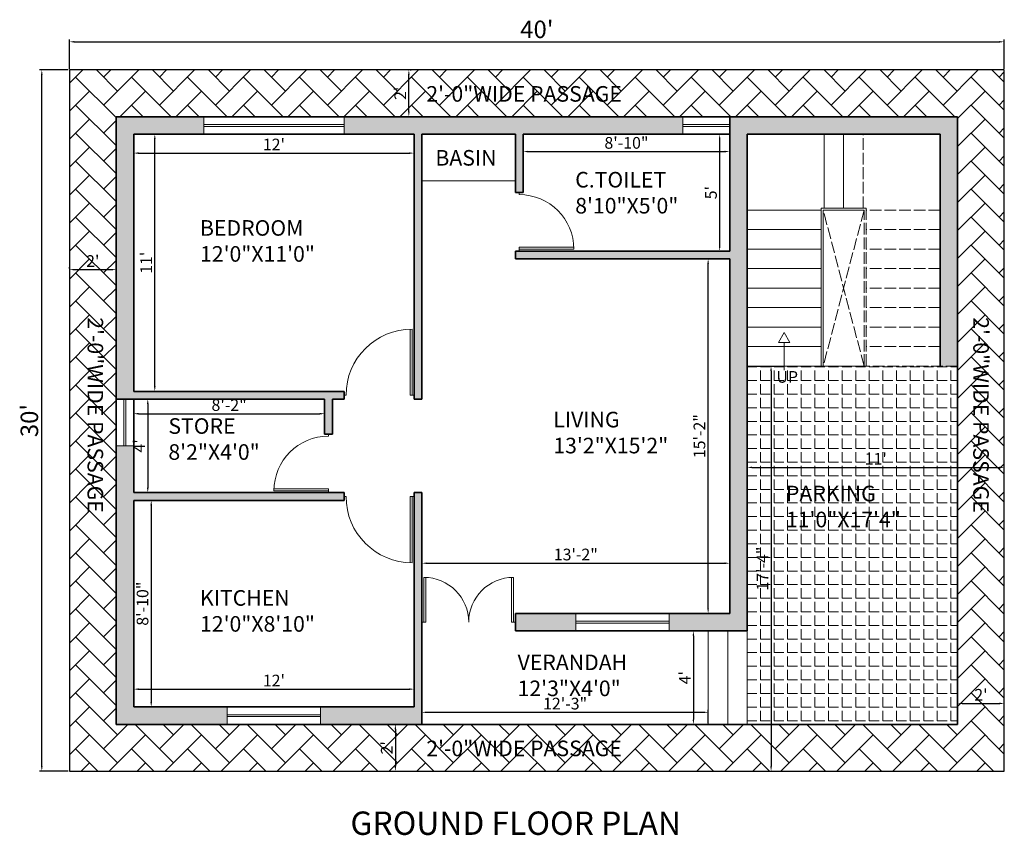
# Model space of a CAD drawing. Units: inches. Extents: x 1947 to 4744, y 610 to 1869.
# Tile 8 of 8: x 4239 to 4744, y 1450 to 1869. Entities that reach past the tile are written whole.
import ezdxf

# ---------------------------------------------------------------- set-up
doc = ezdxf.new("R2010")
doc.units = ezdxf.units.IN
doc.linetypes.add('ACAD_ISO02W100', pattern=[15, 12, -3])
for name, color, linetype, lineweight in [('A-ANNO-DIMS', 2, 'Continuous', 18), ('A-ANNO-SYMB', 2, 'Continuous', 18), ('A-ANNO-TEXT', 7, 'Continuous', 18), ('A-ANNO-TITL', 7, 'Continuous', 35), ('A-AREA-IDEN', 7, 'Continuous', 18), ('A-DOOR', 3, 'Continuous', 18), ('A-FLOR-FIXT', 9, 'Continuous', 18), ('A-FLOR-STRS', 7, 'Continuous', 18), ('A-FLOR-STRS-OVHD', 7, 'ACAD_ISO02W100', 13), ('A-GLAZ', 4, 'Continuous', 18), ('A-WALL', 7, 'Continuous', 35), ('C-PROP', 8, 'Continuous', 25)]:
    doc.layers.add(name, color=color, linetype=linetype, lineweight=lineweight)
doc.layers.add('A-FLOR-PATT', color=251, linetype='Continuous', lineweight=13, true_color=0x636466)
doc.layers.add('A-WALL-PATT', color=18, linetype='Continuous', lineweight=13, true_color=0x000000)
doc.styles.get("Standard").update_dxf_attribs({"font": 'arial.ttf'})
doc.dimstyles.new('ISO-25', dxfattribs={"dimtxt": 9, "dimasz": 2.5, "dimexe": 1.25, "dimexo": 0.625, "dimtad": 1, "dimdec": 1, "dimlunit": 3, "dimtxsty": 'Standard', "dimcen": 2.5, "dimadec": 0, "dimazin": 0, "dimtfac": 1, "dimtdec": 1, "dimtmove": 0, "dimatfit": 3, "dimfxl": 1, "dimarcsym": 0})

# ---------------------------------------------------------------- blocks, each defined once
blk = doc.blocks.new('1')
for p, q in [((4267.36, 1627.82), (4267.36, 1650.82)), ((4268.36, 1627.82), (4268.36, 1650.82)), ((4312.36, 1627.82), (4312.36, 1650.82)), ((4313.36, 1627.82), (4313.36, 1650.82)), ((4266.36, 1627.82), (4268.36, 1627.82)), ((4314.36, 1627.82), (4312.36, 1627.82))]:
    blk.add_line(p, q)
at = {"ltscale": 0.5}
for centre, start, end in [((4267.36, 1627.82), 0, 90), ((4313.36, 1627.82), 90, 180)]:
    blk.add_arc(centre, 23, start, end, dxfattribs=at)
blk = doc.blocks.new('2')
for p, q in [((4319.45, 1679.18), (4319.45, 1713.18)), ((4320.45, 1679.18), (4320.45, 1713.18)), ((4318.45, 1679.18), (4320.45, 1679.18)), ((4353.45, 1679.18), (4354.45, 1679.18))]:
    blk.add_line(p, q)
at = {"ltscale": 0.5}
blk.add_arc((4319.45, 1679.18), 34, 0, 90, dxfattribs=at)
blk = doc.blocks.new('4')
for p, q in [((3808.6, 1693.11), (3808.6, 1721.11)), ((3809.6, 1693.11), (3809.6, 1721.11)), ((3807.6, 1693.11), (3809.6, 1693.11)), ((3836.6, 1693.11), (3837.6, 1693.11))]:
    blk.add_line(p, q)
at = {"ltscale": 0.5}
blk.add_arc((3808.6, 1693.11), 28, 0, 90, dxfattribs=at)
blk = doc.blocks.new('*D11')
at = {"layer": 'A-ANNO-DIMS', "color": 0, "lineweight": -2, "transparency": 16777216}
for p, q in [((4263.57, 1842.83), (4248.77, 1842.83)), ((4250.02, 1485.33), (4250.02, 1840.33)), ((4263.57, 1482.83), (4248.77, 1482.83))]:
    blk.add_line(p, q, dxfattribs=at)
at = {"layer": 'A-ANNO-DIMS', "color": 0, "transparency": 16777216}
for points in [[(4249.6, 1840.33), (4250.44, 1840.33), (4250.02, 1842.83)], [(4249.6, 1485.33), (4250.44, 1485.33), (4250.02, 1482.83)]]:
    blk.add_solid(points, dxfattribs=at)
at = {"layer": 'Defpoints', "color": 0, "transparency": 16777216}
for p in [(4250.02, 1842.83), (4264.19, 1842.83), (4264.19, 1482.83)]:
    blk.add_point(p, dxfattribs=at)
at = {"layer": 'A-ANNO-DIMS', "color": 0, "transparency": 16777216, "insert": (4244.8, 1662.83), "char_height": 9, "attachment_point": 5, "rotation": 90}
blk.add_mtext("30'", dxfattribs=at)
blk = doc.blocks.new('*D12')
at = {"layer": 'A-ANNO-DIMS', "color": 0, "lineweight": -2, "transparency": 16777216}
for p, q in [((4264.19, 1843.45), (4264.19, 1858.52)), ((4266.69, 1857.27), (4741.69, 1857.27)), ((4744.19, 1843.45), (4744.19, 1858.52))]:
    blk.add_line(p, q, dxfattribs=at)
at = {"layer": 'A-ANNO-DIMS', "color": 0, "transparency": 16777216}
for points in [[(4266.69, 1857.68), (4266.69, 1856.85), (4264.19, 1857.27)], [(4741.69, 1857.68), (4741.69, 1856.85), (4744.19, 1857.27)]]:
    blk.add_solid(points, dxfattribs=at)
at = {"layer": 'Defpoints', "color": 0, "transparency": 16777216}
for p in [(4744.19, 1857.27), (4264.19, 1842.83), (4744.19, 1842.83)]:
    blk.add_point(p, dxfattribs=at)
at = {"layer": 'A-ANNO-DIMS', "color": 0, "transparency": 16777216, "insert": (4504.19, 1862.49), "char_height": 9, "attachment_point": 5}
blk.add_mtext("40'", dxfattribs=at)
blk = doc.blocks.new('*D17')
at = {"layer": 'A-ANNO-DIMS', "color": 0, "lineweight": -2, "transparency": 16777216}
for p, q in [((4297.82, 1809.83), (4309.28, 1809.83)), ((4308.03, 1680.33), (4308.03, 1807.33)), ((4297.82, 1677.83), (4309.28, 1677.83))]:
    blk.add_line(p, q, dxfattribs=at)
at = {"layer": 'A-ANNO-DIMS', "color": 0, "transparency": 16777216}
for points in [[(4307.62, 1807.33), (4308.45, 1807.33), (4308.03, 1809.83)], [(4307.62, 1680.33), (4308.45, 1680.33), (4308.03, 1677.83)]]:
    blk.add_solid(points, dxfattribs=at)
at = {"layer": 'Defpoints', "color": 0, "transparency": 16777216}
for p in [(4297.19, 1809.83), (4308.03, 1809.83), (4297.19, 1677.83)]:
    blk.add_point(p, dxfattribs=at)
at = {"layer": 'A-ANNO-DIMS', "color": 0, "transparency": 16777216, "insert": (4304.4, 1743.83), "char_height": 6, "attachment_point": 5, "rotation": 90}
blk.add_mtext("11'", dxfattribs=at)
blk = doc.blocks.new('*D18')
at = {"layer": 'A-ANNO-DIMS', "color": 0, "lineweight": -2, "transparency": 16777216}
for p, q in [((4297.19, 1809.2), (4297.19, 1798.88)), ((4441.19, 1809.2), (4441.19, 1798.88)), ((4299.69, 1800.13), (4438.69, 1800.13))]:
    blk.add_line(p, q, dxfattribs=at)
at = {"layer": 'A-ANNO-DIMS', "color": 0, "transparency": 16777216}
for points in [[(4299.69, 1800.54), (4299.69, 1799.71), (4297.19, 1800.13)], [(4438.69, 1800.54), (4438.69, 1799.71), (4441.19, 1800.13)]]:
    blk.add_solid(points, dxfattribs=at)
at = {"layer": 'Defpoints', "color": 0, "transparency": 16777216}
for p in [(4297.19, 1809.83), (4441.19, 1809.83), (4441.19, 1800.13)]:
    blk.add_point(p, dxfattribs=at)
at = {"layer": 'A-ANNO-DIMS', "color": 0, "transparency": 16777216, "insert": (4369.19, 1803.76), "char_height": 6, "attachment_point": 5}
blk.add_mtext("12'", dxfattribs=at)
blk = doc.blocks.new('*D19')
at = {"layer": 'A-ANNO-DIMS', "color": 0, "lineweight": -2, "transparency": 16777216}
for p, q in [((4497.19, 1809.2), (4497.19, 1799.67)), ((4603.19, 1809.2), (4603.19, 1799.67)), ((4499.69, 1800.92), (4600.69, 1800.92))]:
    blk.add_line(p, q, dxfattribs=at)
at = {"layer": 'A-ANNO-DIMS', "color": 0, "transparency": 16777216}
for points in [[(4499.69, 1801.34), (4499.69, 1800.5), (4497.19, 1800.92)], [(4600.69, 1801.34), (4600.69, 1800.5), (4603.19, 1800.92)]]:
    blk.add_solid(points, dxfattribs=at)
at = {"layer": 'Defpoints', "color": 0, "transparency": 16777216}
for p in [(4497.19, 1809.83), (4603.19, 1809.83), (4603.19, 1800.92)]:
    blk.add_point(p, dxfattribs=at)
at = {"layer": 'A-ANNO-DIMS', "color": 0, "transparency": 16777216, "insert": (4550.19, 1804.61), "char_height": 6, "attachment_point": 5}
blk.add_mtext('8\'-10"', dxfattribs=at)
blk = doc.blocks.new('*D20')
at = {"layer": 'A-ANNO-DIMS', "color": 0, "lineweight": -2, "transparency": 16777216}
for p, q in [((4602.57, 1809.83), (4596.8, 1809.83)), ((4598.05, 1807.33), (4598.05, 1752.33)), ((4602.57, 1749.83), (4596.8, 1749.83))]:
    blk.add_line(p, q, dxfattribs=at)
at = {"layer": 'A-ANNO-DIMS', "color": 0, "transparency": 16777216}
for points in [[(4597.63, 1807.33), (4598.46, 1807.33), (4598.05, 1809.83)], [(4597.63, 1752.33), (4598.46, 1752.33), (4598.05, 1749.83)]]:
    blk.add_solid(points, dxfattribs=at)
at = {"layer": 'Defpoints', "color": 0, "transparency": 16777216}
for p in [(4603.19, 1809.83), (4598.05, 1749.83), (4603.19, 1749.83)]:
    blk.add_point(p, dxfattribs=at)
at = {"layer": 'A-ANNO-DIMS', "color": 0, "transparency": 16777216, "insert": (4594.37, 1779.83), "char_height": 6, "attachment_point": 5, "rotation": 90}
blk.add_mtext("5'", dxfattribs=at)
blk = doc.blocks.new('*D21')
at = {"layer": 'A-ANNO-DIMS', "color": 0, "lineweight": -2, "transparency": 16777216}
for p, q in [((4297.82, 1673.83), (4305.68, 1673.83)), ((4304.43, 1671.33), (4304.43, 1628.33)), ((4297.82, 1625.83), (4305.68, 1625.83))]:
    blk.add_line(p, q, dxfattribs=at)
at = {"layer": 'A-ANNO-DIMS', "color": 0, "transparency": 16777216}
for points in [[(4304.01, 1671.33), (4304.85, 1671.33), (4304.43, 1673.83)], [(4304.01, 1628.33), (4304.85, 1628.33), (4304.43, 1625.83)]]:
    blk.add_solid(points, dxfattribs=at)
at = {"layer": 'Defpoints', "color": 0, "transparency": 16777216}
for p in [(4297.19, 1673.83), (4297.19, 1625.83), (4304.43, 1625.83)]:
    blk.add_point(p, dxfattribs=at)
at = {"layer": 'A-ANNO-DIMS', "color": 0, "transparency": 16777216, "insert": (4300.8, 1649.83), "char_height": 6, "attachment_point": 5, "rotation": 90}
blk.add_mtext("4'", dxfattribs=at)
blk = doc.blocks.new('*D22')
at = {"layer": 'A-ANNO-DIMS', "color": 0, "lineweight": -2, "transparency": 16777216}
for p, q in [((4297.19, 1673.2), (4297.19, 1665.09)), ((4395.19, 1673.2), (4395.19, 1665.09)), ((4299.69, 1666.34), (4392.69, 1666.34))]:
    blk.add_line(p, q, dxfattribs=at)
at = {"layer": 'A-ANNO-DIMS', "color": 0, "transparency": 16777216}
for points in [[(4299.69, 1666.76), (4299.69, 1665.93), (4297.19, 1666.34)], [(4392.69, 1666.76), (4392.69, 1665.93), (4395.19, 1666.34)]]:
    blk.add_solid(points, dxfattribs=at)
at = {"layer": 'Defpoints', "color": 0, "transparency": 16777216}
for p in [(4297.19, 1673.83), (4395.19, 1673.83), (4395.19, 1666.34)]:
    blk.add_point(p, dxfattribs=at)
at = {"layer": 'A-ANNO-DIMS', "color": 0, "transparency": 16777216, "insert": (4346.19, 1670.03), "char_height": 6, "attachment_point": 5}
blk.add_mtext('8\'-2"', dxfattribs=at)
blk = doc.blocks.new('*D23')
at = {"layer": 'A-ANNO-DIMS', "color": 0, "lineweight": -2, "transparency": 16777216}
for p, q in [((4297.82, 1621.83), (4307.45, 1621.83)), ((4306.2, 1619.33), (4306.2, 1518.33)), ((4297.82, 1515.83), (4307.45, 1515.83))]:
    blk.add_line(p, q, dxfattribs=at)
at = {"layer": 'A-ANNO-DIMS', "color": 0, "transparency": 16777216}
for points in [[(4305.78, 1619.33), (4306.61, 1619.33), (4306.2, 1621.83)], [(4305.78, 1518.33), (4306.61, 1518.33), (4306.2, 1515.83)]]:
    blk.add_solid(points, dxfattribs=at)
at = {"layer": 'Defpoints', "color": 0, "transparency": 16777216}
for p in [(4297.19, 1621.83), (4297.19, 1515.83), (4306.2, 1515.83)]:
    blk.add_point(p, dxfattribs=at)
at = {"layer": 'A-ANNO-DIMS', "color": 0, "transparency": 16777216, "insert": (4302.51, 1568.83), "char_height": 6, "attachment_point": 5, "rotation": 90}
blk.add_mtext('8\'-10"', dxfattribs=at)
blk = doc.blocks.new('*D24')
at = {"layer": 'A-ANNO-DIMS', "color": 0, "lineweight": -2, "transparency": 16777216}
for p, q in [((4297.19, 1516.45), (4297.19, 1526.2)), ((4299.69, 1524.95), (4438.69, 1524.95)), ((4441.19, 1516.45), (4441.19, 1526.2))]:
    blk.add_line(p, q, dxfattribs=at)
at = {"layer": 'A-ANNO-DIMS', "color": 0, "transparency": 16777216}
for points in [[(4299.69, 1525.37), (4299.69, 1524.53), (4297.19, 1524.95)], [(4438.69, 1525.37), (4438.69, 1524.53), (4441.19, 1524.95)]]:
    blk.add_solid(points, dxfattribs=at)
at = {"layer": 'Defpoints', "color": 0, "transparency": 16777216}
for p in [(4441.19, 1524.95), (4297.19, 1515.83), (4441.19, 1515.83)]:
    blk.add_point(p, dxfattribs=at)
at = {"layer": 'A-ANNO-DIMS', "color": 0, "transparency": 16777216, "insert": (4369.19, 1528.59), "char_height": 6, "attachment_point": 5}
blk.add_mtext("12'", dxfattribs=at)
blk = doc.blocks.new('*D25')
at = {"layer": 'A-ANNO-DIMS', "color": 0, "lineweight": -2, "transparency": 16777216}
for p, q in [((4445.19, 1588.97), (4445.19, 1588.35)), ((4447.69, 1589.6), (4600.69, 1589.6)), ((4603.19, 1590.22), (4603.19, 1590.85))]:
    blk.add_line(p, q, dxfattribs=at)
at = {"layer": 'A-ANNO-DIMS', "color": 0, "transparency": 16777216}
for points in [[(4447.69, 1590.01), (4447.69, 1589.18), (4445.19, 1589.6)], [(4600.69, 1590.01), (4600.69, 1589.18), (4603.19, 1589.6)]]:
    blk.add_solid(points, dxfattribs=at)
at = {"layer": 'Defpoints', "color": 0, "transparency": 16777216}
for p in [(4445.19, 1589.6), (4603.19, 1589.6), (4603.19, 1589.6)]:
    blk.add_point(p, dxfattribs=at)
at = {"layer": 'A-ANNO-DIMS', "color": 0, "transparency": 16777216, "insert": (4524.19, 1593.29), "char_height": 6, "attachment_point": 5}
blk.add_mtext('13\'-2"', dxfattribs=at)
blk = doc.blocks.new('*D26')
at = {"layer": 'A-ANNO-DIMS', "color": 0, "lineweight": -2, "transparency": 16777216}
for p, q in [((4602.57, 1745.83), (4590.88, 1745.83)), ((4592.13, 1566.33), (4592.13, 1743.33)), ((4602.57, 1563.83), (4590.88, 1563.83))]:
    blk.add_line(p, q, dxfattribs=at)
at = {"layer": 'A-ANNO-DIMS', "color": 0, "transparency": 16777216}
for points in [[(4591.71, 1743.33), (4592.54, 1743.33), (4592.13, 1745.83)], [(4591.71, 1566.33), (4592.54, 1566.33), (4592.13, 1563.83)]]:
    blk.add_solid(points, dxfattribs=at)
at = {"layer": 'Defpoints', "color": 0, "transparency": 16777216}
for p in [(4592.13, 1745.83), (4603.19, 1745.83), (4603.19, 1563.83)]:
    blk.add_point(p, dxfattribs=at)
at = {"layer": 'A-ANNO-DIMS', "color": 0, "transparency": 16777216, "insert": (4588.44, 1654.83), "char_height": 6, "attachment_point": 5, "rotation": 90}
blk.add_mtext('15\'-2"', dxfattribs=at)
blk = doc.blocks.new('*D27')
at = {"layer": 'A-ANNO-DIMS', "color": 0, "lineweight": -2, "transparency": 16777216}
for p, q in [((4432.16, 1506.83), (4432.78, 1506.83)), ((4431.53, 1504.33), (4431.53, 1485.33)), ((4432.16, 1482.83), (4432.78, 1482.83))]:
    blk.add_line(p, q, dxfattribs=at)
at = {"layer": 'A-ANNO-DIMS', "color": 0, "transparency": 16777216}
for points in [[(4431.12, 1504.33), (4431.95, 1504.33), (4431.53, 1506.83)], [(4431.12, 1485.33), (4431.95, 1485.33), (4431.53, 1482.83)]]:
    blk.add_solid(points, dxfattribs=at)
at = {"layer": 'Defpoints', "color": 0, "transparency": 16777216}
for p in [(4431.53, 1506.83), (4431.53, 1482.83), (4431.53, 1482.83)]:
    blk.add_point(p, dxfattribs=at)
at = {"layer": 'A-ANNO-DIMS', "color": 0, "transparency": 16777216, "insert": (4427.9, 1494.83), "char_height": 6, "attachment_point": 5, "rotation": 90}
blk.add_mtext("2'", dxfattribs=at)
blk = doc.blocks.new('*D28')
at = {"layer": 'A-ANNO-DIMS', "color": 0, "lineweight": -2, "transparency": 16777216}
for p, q in [((4264.19, 1740.93), (4264.19, 1741.56)), ((4266.69, 1740.31), (4285.69, 1740.31)), ((4288.19, 1740.93), (4288.19, 1741.56))]:
    blk.add_line(p, q, dxfattribs=at)
at = {"layer": 'A-ANNO-DIMS', "color": 0, "transparency": 16777216}
for points in [[(4266.69, 1740.72), (4266.69, 1739.89), (4264.19, 1740.31)], [(4285.69, 1740.72), (4285.69, 1739.89), (4288.19, 1740.31)]]:
    blk.add_solid(points, dxfattribs=at)
at = {"layer": 'Defpoints', "color": 0, "transparency": 16777216}
for p in [(4264.19, 1740.31), (4288.19, 1740.31), (4288.19, 1740.31)]:
    blk.add_point(p, dxfattribs=at)
at = {"layer": 'A-ANNO-DIMS', "color": 0, "transparency": 16777216, "insert": (4276.19, 1743.94), "char_height": 6, "attachment_point": 5}
blk.add_mtext("2'", dxfattribs=at)
blk = doc.blocks.new('*D29')
at = {"layer": 'A-ANNO-DIMS', "color": 0, "lineweight": -2, "transparency": 16777216}
for p, q in [((4438.47, 1821.33), (4438.47, 1840.33)), ((4439.1, 1842.83), (4439.72, 1842.83)), ((4439.1, 1818.83), (4439.72, 1818.83))]:
    blk.add_line(p, q, dxfattribs=at)
at = {"layer": 'A-ANNO-DIMS', "color": 0, "transparency": 16777216}
for points in [[(4438.06, 1840.33), (4438.89, 1840.33), (4438.47, 1842.83)], [(4438.06, 1821.33), (4438.89, 1821.33), (4438.47, 1818.83)]]:
    blk.add_solid(points, dxfattribs=at)
at = {"layer": 'Defpoints', "color": 0, "transparency": 16777216}
for p in [(4438.47, 1842.83), (4438.47, 1842.83), (4438.47, 1818.83)]:
    blk.add_point(p, dxfattribs=at)
at = {"layer": 'A-ANNO-DIMS', "color": 0, "transparency": 16777216, "insert": (4434.84, 1830.83), "char_height": 6, "attachment_point": 5, "rotation": 90}
blk.add_mtext("2'", dxfattribs=at)
blk = doc.blocks.new('*D30')
at = {"layer": 'A-ANNO-DIMS', "color": 0, "lineweight": -2, "transparency": 16777216}
for p, q in [((4612.19, 1639.41), (4612.19, 1640.03)), ((4614.69, 1638.78), (4741.69, 1638.78)), ((4744.19, 1639.41), (4744.19, 1640.03))]:
    blk.add_line(p, q, dxfattribs=at)
at = {"layer": 'A-ANNO-DIMS', "color": 0, "transparency": 16777216}
for points in [[(4614.69, 1639.2), (4614.69, 1638.37), (4612.19, 1638.78)], [(4741.69, 1639.2), (4741.69, 1638.37), (4744.19, 1638.78)]]:
    blk.add_solid(points, dxfattribs=at)
at = {"layer": 'Defpoints', "color": 0, "transparency": 16777216}
for p in [(4612.19, 1638.78), (4744.19, 1638.78), (4744.19, 1638.78)]:
    blk.add_point(p, dxfattribs=at)
at = {"layer": 'A-ANNO-DIMS', "color": 0, "transparency": 16777216, "insert": (4678.19, 1642.42), "char_height": 6, "attachment_point": 5}
blk.add_mtext("11'", dxfattribs=at)
blk = doc.blocks.new('*D31')
at = {"layer": 'A-ANNO-DIMS', "color": 0, "lineweight": -2, "transparency": 16777216}
for p, q in [((4612.82, 1690.83), (4625.69, 1690.83)), ((4624.44, 1688.33), (4624.44, 1485.33)), ((4612.82, 1482.83), (4625.69, 1482.83))]:
    blk.add_line(p, q, dxfattribs=at)
at = {"layer": 'A-ANNO-DIMS', "color": 0, "transparency": 16777216}
for points in [[(4624.02, 1688.33), (4624.85, 1688.33), (4624.44, 1690.83)], [(4624.02, 1485.33), (4624.85, 1485.33), (4624.44, 1482.83)]]:
    blk.add_solid(points, dxfattribs=at)
at = {"layer": 'Defpoints', "color": 0, "transparency": 16777216}
for p in [(4612.19, 1690.83), (4612.19, 1482.83), (4624.44, 1482.83)]:
    blk.add_point(p, dxfattribs=at)
at = {"layer": 'A-ANNO-DIMS', "color": 0, "transparency": 16777216, "insert": (4620.8, 1586.83), "char_height": 6, "attachment_point": 5, "rotation": 90}
blk.add_mtext('17\'-4"', dxfattribs=at)
blk = doc.blocks.new('*D32')
at = {"layer": 'A-ANNO-DIMS', "color": 0, "lineweight": -2, "transparency": 16777216}
for p, q in [((4445.19, 1507.45), (4445.19, 1514.31)), ((4447.69, 1513.06), (4589.69, 1513.06)), ((4592.19, 1507.45), (4592.19, 1514.31))]:
    blk.add_line(p, q, dxfattribs=at)
at = {"layer": 'A-ANNO-DIMS', "color": 0, "transparency": 16777216}
for points in [[(4447.69, 1513.48), (4447.69, 1512.64), (4445.19, 1513.06)], [(4589.69, 1513.48), (4589.69, 1512.64), (4592.19, 1513.06)]]:
    blk.add_solid(points, dxfattribs=at)
at = {"layer": 'Defpoints', "color": 0, "transparency": 16777216}
for p in [(4592.19, 1513.06), (4445.19, 1506.83), (4592.19, 1506.83)]:
    blk.add_point(p, dxfattribs=at)
at = {"layer": 'A-ANNO-DIMS', "color": 0, "transparency": 16777216, "insert": (4518.69, 1516.75), "char_height": 6, "attachment_point": 5}
blk.add_mtext('12\'-3"', dxfattribs=at)
blk = doc.blocks.new('*D33')
at = {"layer": 'A-ANNO-DIMS', "color": 0, "lineweight": -2, "transparency": 16777216}
for p, q in [((4591.57, 1554.83), (4583.31, 1554.83)), ((4584.56, 1552.33), (4584.56, 1509.33)), ((4591.57, 1506.83), (4583.31, 1506.83))]:
    blk.add_line(p, q, dxfattribs=at)
at = {"layer": 'A-ANNO-DIMS', "color": 0, "transparency": 16777216}
for points in [[(4584.14, 1552.33), (4584.98, 1552.33), (4584.56, 1554.83)], [(4584.14, 1509.33), (4584.98, 1509.33), (4584.56, 1506.83)]]:
    blk.add_solid(points, dxfattribs=at)
at = {"layer": 'Defpoints', "color": 0, "transparency": 16777216}
for p in [(4592.19, 1554.83), (4584.56, 1506.83), (4592.19, 1506.83)]:
    blk.add_point(p, dxfattribs=at)
at = {"layer": 'A-ANNO-DIMS', "color": 0, "transparency": 16777216, "insert": (4580.94, 1530.83), "char_height": 6, "attachment_point": 5, "rotation": 90}
blk.add_mtext("4'", dxfattribs=at)
blk = doc.blocks.new('*D34')
at = {"layer": 'A-ANNO-DIMS', "color": 0, "lineweight": -2, "transparency": 16777216}
for p, q in [((4720.19, 1507.45), (4720.19, 1518.86)), ((4722.69, 1517.61), (4741.69, 1517.61)), ((4744.19, 1507.45), (4744.19, 1518.86))]:
    blk.add_line(p, q, dxfattribs=at)
at = {"layer": 'A-ANNO-DIMS', "color": 0, "transparency": 16777216}
for points in [[(4722.69, 1518.03), (4722.69, 1517.19), (4720.19, 1517.61)], [(4741.69, 1518.03), (4741.69, 1517.19), (4744.19, 1517.61)]]:
    blk.add_solid(points, dxfattribs=at)
at = {"layer": 'Defpoints', "color": 0, "transparency": 16777216}
for p in [(4744.19, 1517.61), (4720.19, 1506.83), (4744.19, 1506.83)]:
    blk.add_point(p, dxfattribs=at)
at = {"layer": 'A-ANNO-DIMS', "color": 0, "transparency": 16777216, "insert": (4732.19, 1521.25), "char_height": 6, "attachment_point": 5}
blk.add_mtext("2'", dxfattribs=at)
blk = doc.blocks.new('STAIR-DIRECTION')
blk.add_line((2.91, 14.18), (2.91, 0))
blk.add_lwpolyline([(2.91, 19.23), (0, 14.18), (5.83, 14.18)], close=True)

msp = doc.modelspace()

# ---------------------------------------------------------------- hatches: boundary and pattern name
at = {"layer": 'A-FLOR-PATT'}
h = msp.add_hatch(dxfattribs=at)
h.set_pattern_fill('AR-HBONE', color=256, scale=0.1)
h.set_pattern_definition([(45, (574.662, 0), (0, 14.36841), [30.48, -10.16]), (135, (581.846, 7.184), (1e-15, 14.36841), [30.48, -10.16])])
h.paths.add_polyline_path([(4264.19, 1842.83), (4264.19, 1482.83), (4744.19, 1482.83), (4744.19, 1842.83)])
h.paths.add_polyline_path([(4720.19, 1818.83), (4720.19, 1506.83), (4288.19, 1506.83), (4288.19, 1818.83)], flags=16)
h.paths.add_polyline_path([(4297.19, 1625.83), (4405.19, 1625.83), (4405.19, 1621.83), (4297.19, 1621.83), (4297.19, 1515.83), (4393.19, 1515.83), (4393.19, 1510.83), (4345.19, 1510.83), (4345.19, 1515.83), (4297.19, 1515.83)], flags=0)
h.paths.add_polyline_path([(4651.19, 1770.83), (4672.19, 1770.83), (4672.19, 1690.83), (4661.69, 1730.83), (4651.19, 1690.83)], flags=0)
h.paths.add_polyline_path([(4449.88, 1789.16), (4489.33, 1789.16), (4489.33, 1806.24), (4449.88, 1806.24)], flags=8)
h.paths.add_polyline_path([(4445.18, 1485.98), (4558.18, 1485.98), (4558.18, 1503.06), (4445.18, 1503.06)], flags=24)
h.paths.add_polyline_path([(4268.95, 1718.11), (4268.95, 1605.12), (4286.03, 1605.12), (4286.03, 1718.11)], flags=24)
h.paths.add_polyline_path([(4723.69, 1718.11), (4723.69, 1605.12), (4740.77, 1605.12), (4740.77, 1718.11)], flags=24)
h.paths.add_polyline_path([(4445.18, 1821.98), (4558.18, 1821.98), (4558.18, 1839.06), (4445.18, 1839.06)], flags=24)
h.paths.add_polyline_path([(4490.92, 1516.82), (4562.48, 1516.82), (4562.48, 1547.23), (4490.92, 1547.23)], flags=8)
h.paths.add_polyline_path([(4628.7, 1603.48), (4690.57, 1603.48), (4690.57, 1633.9), (4628.7, 1633.9)], flags=8)
h.paths.add_polyline_path([(4312.27, 1638.13), (4362.35, 1638.13), (4362.35, 1668.55), (4312.27, 1668.55)], flags=8)
h.paths.add_polyline_path([(4521.17, 1764.58), (4577.62, 1764.58), (4577.62, 1795), (4521.17, 1795)], flags=8)
h.paths.add_polyline_path([(4509.26, 1641.45), (4571.13, 1641.45), (4571.13, 1671.86), (4509.26, 1671.86)], flags=8)
h.paths.add_polyline_path([(4327.86, 1549.89), (4389.73, 1549.89), (4389.73, 1580.3), (4327.86, 1580.3)], flags=8)
h.paths.add_polyline_path([(4327.86, 1739.82), (4392.11, 1739.82), (4392.11, 1770.24), (4327.86, 1770.24)], flags=8)
h = msp.add_hatch(dxfattribs=at)
h.set_pattern_fill('ANGLE', color=256)
h.set_pattern_definition([(0, (574.662, 0), (0, 6.985), [5.08, -1.905]), (90, (574.662, 0), (-6.985, 4e-16), [5.08, -1.905])])
h.paths.add_polyline_path([(4720.19, 1690.83), (4672.19, 1690.83), (4612.19, 1690.83), (4612.19, 1554.83), (4612.19, 1506.83), (4720.19, 1506.83)])
h.paths.add_polyline_path([(4625.66, 1678.84), (4639.99, 1678.84), (4639.99, 1691.65), (4625.66, 1691.65)], flags=9)
h.paths.add_polyline_path([(4628.7, 1603.48), (4690.57, 1603.48), (4690.57, 1633.9), (4628.7, 1633.9)], flags=24)
at = {"layer": 'A-WALL-PATT'}
h = msp.add_hatch(color=256, dxfattribs=at)
h.dxf.hatch_style = 1
h.paths.add_polyline_path([(4333.19, 1818.83), (4288.19, 1818.83), (4288.19, 1673.83), (4395.19, 1673.83), (4395.19, 1655.83), (4399.19, 1655.83), (4399.19, 1673.83), (4405.19, 1673.83), (4405.19, 1677.83), (4297.19, 1677.83), (4297.19, 1809.83), (4333.19, 1809.83)])
h.paths.add_polyline_path([(4579.19, 1818.83), (4405.19, 1818.83), (4405.19, 1809.83), (4441.19, 1809.83), (4441.19, 1673.83), (4445.19, 1673.83), (4445.19, 1809.83), (4493.19, 1809.83), (4493.19, 1779.83), (4497.19, 1779.83), (4497.19, 1809.83), (4579.19, 1809.83)])
h.paths.add_polyline_path([(4612.19, 1809.83), (4711.19, 1809.83), (4711.19, 1690.83), (4720.19, 1690.83), (4720.19, 1818.83), (4603.19, 1818.83), (4603.19, 1749.83), (4493.19, 1749.83), (4493.19, 1745.83), (4603.19, 1745.83), (4603.19, 1563.83), (4572.19, 1563.83), (4572.19, 1554.83), (4612.19, 1554.83)])
h.paths.add_polyline_path([(4445.19, 1625.83), (4441.19, 1625.83), (4441.19, 1515.83), (4393.19, 1515.83), (4393.19, 1506.83), (4445.19, 1506.83)])
h.paths.add_polyline_path([(4345.19, 1515.83), (4297.19, 1515.83), (4297.19, 1621.83), (4405.19, 1621.83), (4405.19, 1625.83), (4297.19, 1625.83), (4297.19, 1649.83), (4288.19, 1649.83), (4288.19, 1506.83), (4345.19, 1506.83)])
h.paths.add_polyline_path([(4524.19, 1563.83), (4493.19, 1563.83), (4493.19, 1554.83), (4524.19, 1554.83)])

# ---------------------------------------------------------------- linework, layer by layer
at = {"layer": 'A-FLOR-FIXT'}
msp.add_line((4493.19, 1785.83), (4445.19, 1785.83), dxfattribs=at)
at = {"layer": 'A-FLOR-STRS'}
for p, q in [((4651.69, 1771.83), (4651.69, 1809.83)), ((4661.69, 1771.83), (4661.69, 1809.83)), ((4650.19, 1770.83), (4612.19, 1770.83)), ((4673.19, 1771.83), (4650.19, 1771.83)), ((4650.19, 1690.83), (4650.19, 1771.83)), ((4672.19, 1770.83), (4651.19, 1770.83)), ((4651.19, 1690.83), (4651.19, 1770.83)), ((4650.19, 1760.83), (4612.19, 1760.83)), ((4650.19, 1750.83), (4612.19, 1750.83)), ((4650.19, 1740.83), (4612.19, 1740.83)), ((4650.19, 1730.83), (4612.19, 1730.83)), ((4650.19, 1720.83), (4612.19, 1720.83)), ((4650.19, 1710.83), (4612.19, 1710.83)), ((4650.19, 1700.83), (4612.19, 1700.83)), ((4672.19, 1690.83), (4612.19, 1690.83)), ((4592.19, 1554.83), (4592.19, 1506.83)), ((4602.19, 1554.83), (4602.19, 1506.83)), ((4612.19, 1554.83), (4612.19, 1506.83))]:
    msp.add_line(p, q, dxfattribs=at)
at = {"layer": 'A-FLOR-STRS-OVHD', "ltscale": 0.5}
for p, q in [((4671.69, 1771.83), (4671.69, 1809.83)), ((4672.19, 1770.83), (4651.19, 1690.83)), ((4672.19, 1690.83), (4651.19, 1770.83)), ((4672.19, 1690.83), (4672.19, 1770.83)), ((4673.19, 1690.83), (4673.19, 1771.83)), ((4711.19, 1770.83), (4673.19, 1770.83)), ((4711.19, 1760.83), (4673.19, 1760.83)), ((4711.19, 1750.83), (4673.19, 1750.83)), ((4711.19, 1740.83), (4673.19, 1740.83)), ((4711.19, 1730.83), (4673.19, 1730.83)), ((4711.19, 1720.83), (4673.19, 1720.83)), ((4711.19, 1710.83), (4673.19, 1710.83)), ((4711.19, 1700.83), (4673.19, 1700.83)), ((4720.19, 1690.83), (4672.19, 1690.83))]:
    msp.add_line(p, q, dxfattribs=at)
at = {"layer": 'A-GLAZ'}
for p, q in [((4333.19, 1809.83), (4333.19, 1818.83)), ((4405.19, 1809.83), (4405.19, 1818.83)), ((4579.19, 1809.83), (4579.19, 1818.83)), ((4405.19, 1814.83), (4333.19, 1814.83)), ((4405.19, 1813.83), (4333.19, 1813.83)), ((4603.19, 1814.83), (4579.19, 1814.83)), ((4603.19, 1813.83), (4579.19, 1813.83)), ((4292.19, 1673.83), (4292.19, 1649.83)), ((4293.19, 1673.83), (4293.19, 1649.83)), ((4297.19, 1649.83), (4288.19, 1649.83)), ((4524.19, 1554.83), (4524.19, 1563.83)), ((4572.19, 1554.83), (4572.19, 1563.83)), ((4572.19, 1559.83), (4524.19, 1559.83)), ((4572.19, 1558.83), (4524.19, 1558.83)), ((4345.19, 1506.83), (4345.19, 1515.83)), ((4393.19, 1511.83), (4345.19, 1511.83)), ((4393.19, 1506.83), (4393.19, 1515.83)), ((4393.19, 1510.83), (4345.19, 1510.83))]:
    msp.add_line(p, q, dxfattribs=at)
at = {"layer": 'A-WALL'}
for p, q in [((4720.19, 1818.83), (4288.19, 1818.83)), ((4288.19, 1818.83), (4288.19, 1506.83)), ((4603.19, 1749.83), (4603.19, 1818.83)), ((4720.19, 1506.83), (4720.19, 1818.83)), ((4441.19, 1809.83), (4297.19, 1809.83)), ((4297.19, 1809.83), (4297.19, 1677.83)), ((4441.19, 1809.83), (4441.19, 1673.83)), ((4493.19, 1809.83), (4445.19, 1809.83)), ((4445.19, 1809.83), (4445.19, 1673.83)), ((4493.19, 1779.83), (4493.19, 1809.83)), ((4603.19, 1809.83), (4497.19, 1809.83)), ((4497.19, 1779.83), (4497.19, 1809.83)), ((4711.19, 1809.83), (4612.19, 1809.83)), ((4612.19, 1554.83), (4612.19, 1809.83)), ((4711.19, 1690.83), (4711.19, 1809.83)), ((4497.19, 1779.83), (4493.19, 1779.83)), ((4603.19, 1749.83), (4493.19, 1749.83)), ((4493.19, 1745.83), (4493.19, 1749.83)), ((4493.19, 1745.83), (4603.19, 1745.83)), ((4603.19, 1563.83), (4603.19, 1745.83)), ((4395.19, 1673.83), (4288.19, 1673.83)), ((4405.19, 1677.83), (4297.19, 1677.83)), ((4297.19, 1673.83), (4297.19, 1625.83)), ((4395.19, 1673.83), (4395.19, 1655.83)), ((4405.19, 1673.83), (4399.19, 1673.83)), ((4399.19, 1673.83), (4399.19, 1655.83)), ((4405.19, 1677.83), (4405.19, 1673.83)), ((4445.19, 1673.83), (4441.19, 1673.83)), ((4399.19, 1655.83), (4395.19, 1655.83)), ((4405.19, 1625.83), (4297.19, 1625.83)), ((4405.19, 1625.83), (4405.19, 1621.83)), ((4445.19, 1625.83), (4441.19, 1625.83)), ((4441.19, 1625.83), (4441.19, 1515.83)), ((4445.19, 1625.83), (4445.19, 1506.83)), ((4405.19, 1621.83), (4297.19, 1621.83)), ((4297.19, 1621.83), (4297.19, 1515.83)), ((4493.19, 1563.83), (4493.19, 1554.83)), ((4493.19, 1563.83), (4603.19, 1563.83)), ((4493.19, 1554.83), (4612.19, 1554.83)), ((4297.19, 1515.83), (4441.19, 1515.83)), ((4288.19, 1506.83), (4720.19, 1506.83))]:
    msp.add_line(p, q, dxfattribs=at)
at = {"layer": 'C-PROP'}
msp.add_lwpolyline([(4264.19, 1482.83), (4744.19, 1482.83), (4744.19, 1842.83), (4264.19, 1842.83)], close=True, dxfattribs=at)

# ---------------------------------------------------------------- block references
at = {"layer": 'A-ANNO-SYMB'}
msp.add_blockref('STAIR-DIRECTION', (4628.28, 1688.75), dxfattribs=at)
at = {"layer": 'A-DOOR', "xscale": -1, "rotation": 270}
msp.add_blockref('4', (2802.08, -2057.77), dxfattribs=at)
at = {"layer": 'A-DOOR', "xscale": -1}
msp.add_blockref('2', (8759.65, -3.36), dxfattribs=at)
at = {"layer": 'A-DOOR'}
for name, p, rotation in [('4', (6090.3, -2181.77), 90), ('2', (8759.65, 3303.01), 180)]:
    msp.add_blockref(name, p, dxfattribs=dict(at, rotation=rotation))
msp.add_blockref('1', (178.83, -68.5), dxfattribs=at)

# ---------------------------------------------------------------- texts
at = {"layer": 'A-ANNO-TEXT', "attachment_point": 1}
for s, insert, char_height in [('{\\fTimes New Roman|b0|i0|c0|p18;BASIN}', (4452.08, 1801.71), 8), ('{\\fTimes New Roman|b0|i0|c0|p18;UP}', (4627.21, 1688.25), 6)]:
    msp.add_mtext_dynamic_manual_height_columns(s, width=158.3328, gutter_width=12.5, heights=[0], dxfattribs=dict(at, insert=insert, char_height=char_height))
at = {"layer": 'A-ANNO-TITL', "insert": (4408.49, 1462.13), "char_height": 12, "attachment_point": 1}
msp.add_mtext_dynamic_manual_height_columns('{\\fTimes New Roman|b0|i0|c0|p18;GROUND FLOOR PLAN}', width=253.4596, gutter_width=12.5, heights=[0], dxfattribs=at)
at = {"layer": 'A-AREA-IDEN', "char_height": 8, "attachment_point": 1}
for s, width, heights, insert in [('{\\fTimes New Roman|b0|i0|c0|p18;2\'-0"WIDE PASSAGE}', 158.3328, [0], (4447.44, 1834.53)), ('{\\fTimes New Roman|b0|i0|c0|p18;C.TOILET\\P8\'10"X5\'0"}', 64.3566, [21.47], (4523.89, 1790.47)), ('{\\fTimes New Roman|b0|i0|c0|p18;BEDROOM\\P12\'0"X11\'0"}', 64.3566, [0], (4331.24, 1765.71)), ('{\\fTimes New Roman|b0|i0|c0|p18;STORE\\P8\'2"X4\'0"}', 64.3566, [21.47], (4315.01, 1664.02)), ('{\\fTimes New Roman|b0|i0|c0|p18;LIVING\\P13\'2"X15\'2"}', 64.3566, [21.47], (4512.64, 1667.33)), ('{\\fTimes New Roman|b0|i0|c0|p18;PARKING\\P11\'0"X17\'4"}', 64.3566, [0], (4632.08, 1629.37)), ('{\\fTimes New Roman|b0|i0|c0|p18;KITCHEN\\P12\'0"X8\'10"}', 64.3566, [0], (4331.24, 1575.78)), ('{\\fTimes New Roman|b0|i0|c0|p18;VERANDAH\\P12\'3"X4\'0"}', 64.3566, [0], (4494.3, 1542.7)), ('{\\fTimes New Roman|b0|i0|c0|p18;2\'-0"WIDE PASSAGE}', 158.3328, [0], (4447.44, 1498.53))]:
    msp.add_mtext_dynamic_manual_height_columns(s, width=width, gutter_width=12.5, heights=heights, dxfattribs=dict(at, insert=insert))
at = {"layer": 'A-AREA-IDEN', "char_height": 8, "attachment_point": 1, "rotation": 270}
for insert in [(4281.5, 1715.86), (4736.24, 1715.86)]:
    msp.add_mtext_dynamic_manual_height_columns('{\\fTimes New Roman|b0|i0|c0|p18;2\'-0"WIDE PASSAGE}', width=158.3328, gutter_width=12.5, heights=[0], dxfattribs=dict(at, insert=insert))

# ---------------------------------------------------------------- dimensions: what is measured, and where the dimension line sits
at = {"layer": 'A-ANNO-DIMS'}
for base, p1, p2, override, picture, middle in [((4744.19, 1857.27), (4264.19, 1842.83), (4744.19, 1842.83), {"dimclrd": 0, "dimclre": 0, "dimclrt": 0}, '*D12', (4504.19, 1862.49)), ((4441.19, 1800.13), (4297.19, 1809.83), (4441.19, 1809.83), {"dimtxt": 6, "dimclrd": 0, "dimclre": 0, "dimclrt": 0}, '*D18', (4369.19, 1803.76)), ((4603.19, 1800.92), (4497.19, 1809.83), (4603.19, 1809.83), {"dimtxt": 6, "dimclrd": 0, "dimclre": 0, "dimclrt": 0}, '*D19', (4550.19, 1804.61)), ((4288.19, 1740.31), (4264.19, 1740.31), (4288.19, 1740.31), {"dimtxt": 6, "dimclrd": 0, "dimclre": 0, "dimclrt": 0}, '*D28', (4276.19, 1743.94)), ((4395.19, 1666.34), (4297.19, 1673.83), (4395.19, 1673.83), {"dimtxt": 6, "dimclrd": 0, "dimclre": 0, "dimclrt": 0}, '*D22', (4346.19, 1670.03)), ((4744.19, 1638.78), (4612.19, 1638.78), (4744.19, 1638.78), {"dimtxt": 6, "dimclrd": 0, "dimclre": 0, "dimclrt": 0}, '*D30', (4678.19, 1642.42)), ((4603.19, 1589.6), (4445.19, 1589.6), (4603.19, 1589.6), {"dimtxt": 6, "dimclrd": 0, "dimclre": 0, "dimclrt": 0}, '*D25', (4524.19, 1593.29)), ((4441.19, 1524.95), (4297.19, 1515.83), (4441.19, 1515.83), {"dimtxt": 6, "dimclrd": 0, "dimclre": 0, "dimclrt": 0}, '*D24', (4369.19, 1528.59)), ((4744.19, 1517.61), (4720.19, 1506.83), (4744.19, 1506.83), {"dimtxt": 6, "dimclrd": 0, "dimclre": 0, "dimclrt": 0}, '*D34', (4732.19, 1521.25)), ((4592.19, 1513.06), (4445.19, 1506.83), (4592.19, 1506.83), {"dimtxt": 6, "dimclrd": 0, "dimclre": 0, "dimclrt": 0}, '*D32', (4518.69, 1516.75))]:
    dim = msp.add_linear_dim(base=base, p1=p1, p2=p2, dimstyle='ISO-25', override=override, dxfattribs=at)
    dim.commit()
    dim.dimension.update_dxf_attribs({"geometry": picture, "text_midpoint": middle})
for base, p1, p2, angle, override, picture, middle in [((4250.02, 1842.83), (4264.19, 1482.83), (4264.19, 1842.83), 90, {"dimclrd": 0, "dimclre": 0, "dimclrt": 0}, '*D11', (4244.8, 1662.83)), ((4438.47, 1842.83), (4438.47, 1818.83), (4438.47, 1842.83), 90, {"dimtxt": 6, "dimclrd": 0, "dimclre": 0, "dimclrt": 0}, '*D29', (4434.84, 1830.83)), ((4308.03, 1809.83), (4297.19, 1677.83), (4297.19, 1809.83), 270, {"dimtxt": 6, "dimclrd": 0, "dimclre": 0, "dimclrt": 0}, '*D17', (4304.4, 1743.83)), ((4598.05, 1749.83), (4603.19, 1809.83), (4603.19, 1749.83), 90, {"dimtxt": 6, "dimclrd": 0, "dimclre": 0, "dimclrt": 0}, '*D20', (4594.37, 1779.83)), ((4592.13, 1745.83), (4603.19, 1563.83), (4603.19, 1745.83), 90, {"dimtxt": 6, "dimclrd": 0, "dimclre": 0, "dimclrt": 0}, '*D26', (4588.44, 1654.83)), ((4624.44, 1482.83), (4612.19, 1690.83), (4612.19, 1482.83), 90, {"dimtxt": 6, "dimclrd": 0, "dimclre": 0, "dimclrt": 0}, '*D31', (4620.8, 1586.83)), ((4304.43, 1625.83), (4297.19, 1673.83), (4297.19, 1625.83), 90, {"dimtxt": 6, "dimclrd": 0, "dimclre": 0, "dimclrt": 0}, '*D21', (4300.8, 1649.83)), ((4306.2, 1515.83), (4297.19, 1621.83), (4297.19, 1515.83), 90, {"dimtxt": 6, "dimclrd": 0, "dimclre": 0, "dimclrt": 0}, '*D23', (4302.51, 1568.83)), ((4584.56, 1506.83), (4592.19, 1554.83), (4592.19, 1506.83), 90, {"dimtxt": 6, "dimclrd": 0, "dimclre": 0, "dimclrt": 0}, '*D33', (4580.94, 1530.83)), ((4431.53, 1482.83), (4431.53, 1506.83), (4431.53, 1482.83), 90, {"dimtxt": 6, "dimclrd": 0, "dimclre": 0, "dimclrt": 0}, '*D27', (4427.9, 1494.83))]:
    dim = msp.add_linear_dim(base=base, p1=p1, p2=p2, angle=angle, dimstyle='ISO-25', override=override, dxfattribs=at)
    dim.commit()
    dim.dimension.update_dxf_attribs({"geometry": picture, "text_midpoint": middle})

doc.saveas('drawing.dxf')
